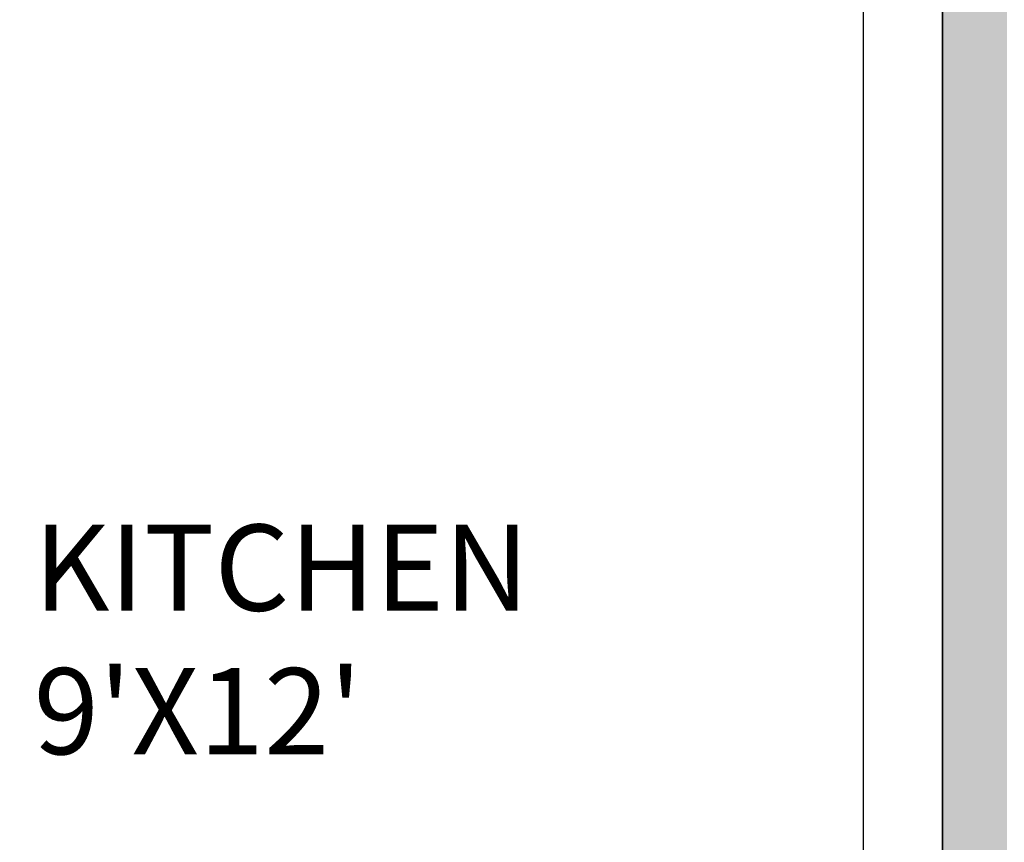
# Model space of a CAD drawing. Units: inches. Extents: x -5 to 482, y -460 to 66.
# Tile 22 of 31: x 86 to 154, y -86 to -29. Entities that reach past the tile are written whole.
import ezdxf

# ---------------------------------------------------------------- set-up
doc = ezdxf.new("R2010")
doc.units = ezdxf.units.IN
doc.header["$MEASUREMENT"] = 0
for name, color, linetype, lineweight in [('A-ANNO-DIMS', 2, 'Continuous', 18), ('A-AREA-IDEN', 7, 'Continuous', 18), ('A-WALL', 7, 'Continuous', 35), ('A-WALL-PATT', 152, 'Continuous', 13)]:
    doc.layers.add(name, color=color, linetype=linetype, lineweight=lineweight)
doc.styles.get("Standard").update_dxf_attribs({"font": 'arial.ttf'})
doc.dimstyles.get("Standard").update_dxf_attribs({"dimtxt": 0.18, "dimasz": 0.18, "dimexe": 0.18, "dimexo": 0.0625, "dimgap": 0.09, "dimtad": 0, "dimtih": 1, "dimtoh": 1, "dimdec": 0, "dimzin": 0, "dimdsep": 46, "dimlunit": 3, "dimtxsty": 'Standard', "dimcen": 0.09, "dimadec": 0, "dimazin": 0, "dimtfac": 1, "dimtdec": 0, "dimtofl": 0, "dimtmove": 0, "dimatfit": 3, "dimfxl": 1, "dimtolj": 1, "dimtzin": 0, "dimarcsym": 0})

# ---------------------------------------------------------------- blocks, each defined once
blk = doc.blocks.new('*D73')
at = {"layer": 'A-ANNO-DIMS', "color": 0, "lineweight": -2, "transparency": 16777216}
for p, q in [((144.377, -295.799), (144.377, 50.931)), ((144.557, 50.751), (160.976, 50.751)), ((178.197, 50.751), (161.777, 50.751)), ((178.377, -295.799), (178.377, 50.931))]:
    blk.add_line(p, q, dxfattribs=at)
at = {"layer": 'A-ANNO-DIMS', "color": 0, "transparency": 16777216}
for points in [[(144.557, 50.781), (144.557, 50.721), (144.377, 50.751)], [(178.197, 50.781), (178.197, 50.721), (178.377, 50.751)]]:
    blk.add_solid(points, dxfattribs=at)
at = {"layer": 'Defpoints', "color": 0, "transparency": 16777216}
for p in [(178.377, 50.751), (144.377, -295.861), (178.377, -295.861)]:
    blk.add_point(p, dxfattribs=at)
at = {"layer": 'A-ANNO-DIMS', "color": 0, "transparency": 16777216, "insert": (161.377, 50.751), "char_height": 0.18, "attachment_point": 5}
blk.add_mtext('\\A1;2\'-10"', dxfattribs=at)

msp = doc.modelspace()

# ---------------------------------------------------------------- hatches: boundary and pattern name
at = {"layer": 'A-WALL-PATT'}
h = msp.add_hatch(color=256, dxfattribs=at)
h.dxf.hatch_style = 1
h.paths.add_polyline_path([(149.377, -412.849), (144.377, -412.849), (144.377, -283.849), (144.377, -279.349), (133.877, -279.349), (133.877, -283.849), (139.877, -283.849), (139.877, -412.849), (133.51, -412.849), (133.51, -413.916), (102.652, -413.916), (102.652, -421.02), (133.51, -421.02), (133.51, -421.849), (149.377, -421.849)])
h.paths.add_polyline_path([(226.054, -412.849), (218.877, -412.849), (218.877, -350.849), (262.877, -350.849), (262.877, -386.849), (267.377, -386.849), (267.377, -283.849), (270.377, -283.849), (270.377, -279.349), (244.877, -279.349), (244.877, -283.849), (262.877, -283.849), (262.877, -346.349), (218.877, -346.349), (218.877, -283.849), (220.877, -283.849), (220.877, -279.349), (214.377, -279.349), (214.377, -283.849), (214.377, -412.849), (209.377, -412.849), (209.377, -421.849), (226.054, -421.849)])
h.paths.add_polyline_path([(315.815, -412.849), (250.054, -412.849), (250.054, -421.849), (315.815, -421.849)])
h.paths.add_polyline_path([(430.377, -378.349), (421.377, -378.349), (421.377, -412.849), (375.815, -412.849), (375.815, -421.849), (430.377, -421.849)])
h.paths.add_polyline_path([(78.691, -413.916), (47.68, -413.916), (47.68, -412.849), (41.877, -412.849), (41.877, -283.849), (109.877, -283.849), (109.877, -279.349), (41.877, -279.349), (41.877, -241.849), (32.877, -241.849), (32.877, -421.849), (47.68, -421.849), (47.68, -421.02), (78.691, -421.02)])
h.paths.add_polyline_path([(41.877, -144.349), (154.377, -144.349), (154.377, -137.849), (149.877, -137.849), (149.877, -139.849), (41.877, -139.849), (41.877, -97.849), (32.877, -97.849), (32.877, -181.849), (41.877, -181.849)])
h.paths.add_polyline_path([(430.377, -241.849), (421.377, -241.849), (421.377, -279.349), (309.377, -279.349), (309.377, -170.349), (304.877, -170.349), (304.877, -279.349), (294.377, -279.349), (294.377, -283.849), (421.377, -283.849), (421.377, -318.349), (430.377, -318.349)])
h.paths.add_polyline_path([(430.377, -119.849), (421.377, -119.849), (421.377, -139.849), (419.377, -139.849), (419.377, -144.349), (421.377, -144.349), (421.377, -181.849), (430.377, -181.849)])
h.paths.add_polyline_path([(395.377, -139.849), (377.377, -139.849), (377.377, -75.849), (421.377, -75.849), (421.377, -95.849), (430.377, -95.849), (430.377, -45.599), (421.377, -45.599), (421.377, -71.349), (377.377, -71.349), (377.377, -22.849), (372.877, -22.849), (372.877, -139.849), (242.877, -139.849), (242.877, -137.849), (238.377, -137.849), (238.377, -144.349), (304.877, -144.349), (304.877, -146.349), (309.377, -146.349), (309.377, -144.349), (395.377, -144.349)])
h.paths.add_polyline_path([(65.877, 13.151), (32.877, 13.151), (32.877, -37.849), (41.877, -37.849), (41.877, 4.151), (65.877, 4.151)])
h.paths.add_polyline_path([(166.377, 13.151), (125.877, 13.151), (125.877, 4.151), (149.877, 4.151), (149.877, -113.849), (154.377, -113.849), (154.377, 4.151), (166.377, 4.151)])
h.paths.add_polyline_path([(277.877, 13.151), (226.377, 13.151), (226.377, 4.151), (238.377, 4.151), (238.377, -113.849), (242.877, -113.849), (242.877, 4.151), (277.877, 4.151)])
h.paths.add_polyline_path([(430.377, 13.151), (337.877, 13.151), (337.877, 4.151), (372.877, 4.151), (372.877, 1.151), (377.377, 1.151), (377.377, 4.151), (421.377, 4.151), (421.377, -21.599), (430.377, -21.599)])

# ---------------------------------------------------------------- linework, layer by layer
at = {"layer": 'A-WALL'}
msp.add_line((149.877, 4.151), (149.877, -113.849), dxfattribs=at)

# ---------------------------------------------------------------- texts
at = {"layer": 'A-AREA-IDEN', "insert": (86.59, -63.672), "char_height": 6, "attachment_point": 1}
msp.add_mtext("KITCHEN\\P9'X12'", dxfattribs=at)

# ---------------------------------------------------------------- dimensions: what is measured, and where the dimension line sits
at = {"layer": 'A-ANNO-DIMS'}
dim = msp.add_linear_dim(base=(178.377, 50.751), p1=(144.377, -295.861), p2=(178.377, -295.861), dimstyle='Standard', override={"dimdec": 1, "dimlfac": 1, "dimrnd": 0, "dimzin": 1, "dimdsep": 46, "dimlunit": 4, "dimfrac": 2}, dxfattribs=at)
dim.commit()
dim.dimension.update_dxf_attribs({"geometry": '*D73', "text_midpoint": (161.377, 50.751)})

doc.saveas('drawing.dxf')
